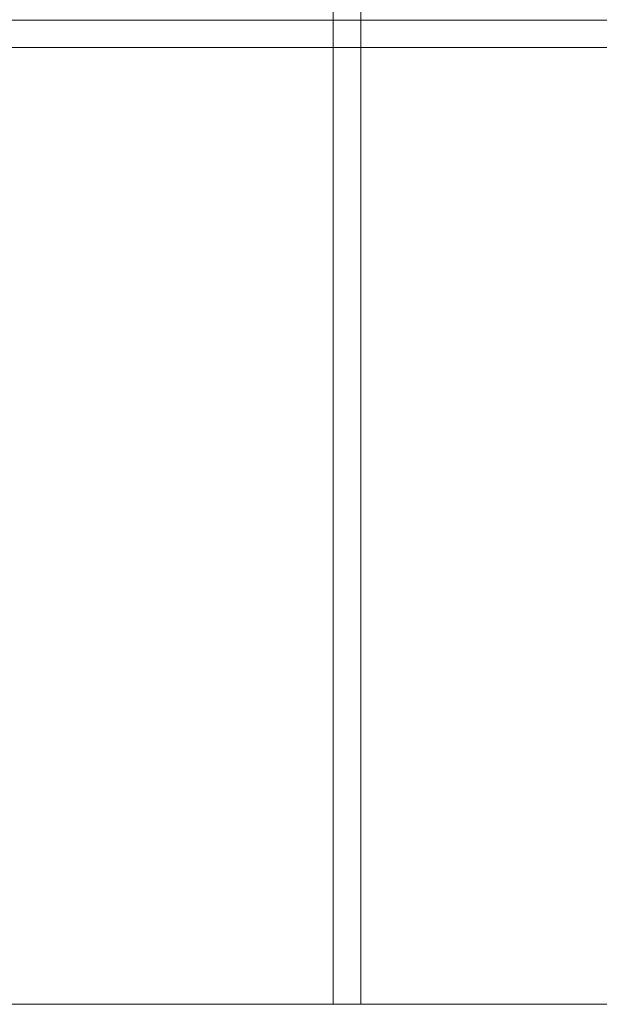
# Model space of a CAD drawing. Units: inches. Extents: x -17 to 1735, y -531 to 60.
# Tile 10 of 27: x 1734.67915 to 1734.69407, y -150.22418 to -150.19886. Entities that reach past the tile are written whole.
import ezdxf

# ---------------------------------------------------------------- set-up
doc = ezdxf.new("R2010")
doc.units = ezdxf.units.IN
doc.header["$MEASUREMENT"] = 0
doc.layers.add('A-FURN', color=242, linetype='Continuous', lineweight=18, true_color=0xcd2027)

# ---------------------------------------------------------------- blocks, each defined once
blk = doc.blocks.new('childrens_room_2')
for p, q in [((70.47533, 55.33419), (70.47533, 53.9594)), ((70.49333, 55.33419), (70.49333, 53.9594)), ((69.75691, 54.60219), (71.20991, 54.60219)), ((69.75691, 54.58419), (71.20991, 54.58419)), ((69.75691, 53.9594), (71.77791, 53.9594))]:
    blk.add_line(p, q)

msp = doc.modelspace()

# ---------------------------------------------------------------- block references
at = {"layer": 'A-FURN', "xscale": 0.0393700787401575, "yscale": 0.0393700787401575, "zscale": 0.0393700787401575}
msp.add_blockref('childrens_room_2', (1731.912601, -152.348565), dxfattribs=at)

doc.saveas('drawing.dxf')
